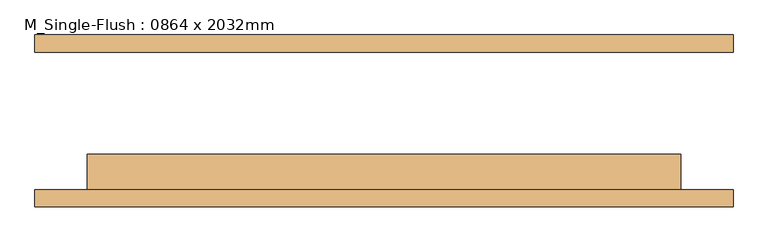
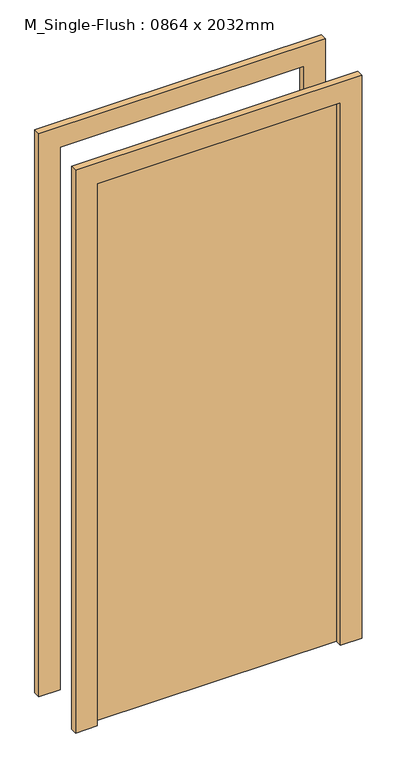
"""IFC4 building model written with IfcOpenShell, lengths in millimetres: door geometry, M_Single-Flush : 0864 x 2032mm."""

from ifc_helpers import new_model, si_unit, frame, origin, origin_with_axes, place, context, project, spatial, polyline, outline, extrude, source, transform, mapped, element, save


def m_single_flush_0864_x_2032mm_0516f16c(model_context):
    return source(origin(), model_context, "Body", "SweptSolid", [
        extrude(outline(polyline([(2108.0, -508.0), (0.0, -508.0), (0.0, -432.0), (2032.0, -432.0), (2032.0, 432.0), (0.0, 432.0), (0.0, 508.0), (2108.0, 508.0), (2108.0, -508.0)])), frame((0.0, -125.0, 0.0), z_axis=(0.0, 1.0, 0.0), x_axis=(0.0, 0.0, 1.0)), (0.0, 0.0, 1.0), 25.0),
        extrude(outline(polyline([(2108.0, 508.0), (2108.0, -508.0), (0.0, -508.0), (0.0, -432.0), (2032.0, -432.0), (2032.0, 432.0), (0.0, 432.0), (0.0, 508.0), (2108.0, 508.0)])), frame((0.0, 100.0, 0.0), z_axis=(0.0, 1.0, 0.0), x_axis=(0.0, 0.0, 1.0)), (0.0, 0.0, 1.0), 25.0),
        extrude(outline(polyline([(432.0, -49.0), (432.0, -100.0), (-432.0, -100.0), (-432.0, -49.0), (432.0, -49.0)])), origin_with_axes(), (0.0, 0.0, 1.0), 2032.0),
    ])


if __name__ == "__main__":
    model = new_model("IFC4")
    model_context = context("Model", 3, world=origin())
    ifc_project = project(units=[si_unit("LENGTHUNIT", "METRE", prefix="MILLI")], contexts=[model_context])
    site = spatial("IfcSite", under=ifc_project)
    building = spatial("IfcBuilding", under=site)
    placement = place(None, origin())
    m_single_flush_0864_x_2032mm_shape = m_single_flush_0864_x_2032mm_0516f16c(model_context)
    element("IfcDoor", 1, ObjectType="M_Single-Flush : 0864 x 2032mm", at=placement, inside=building, context=model_context, shape_type="MappedRepresentation", body=[
        mapped(m_single_flush_0864_x_2032mm_shape, transform((0.0, 0.0, 0.0), x_axis=(1.0, 0.0, 0.0), y_axis=(0.0, 1.0, 0.0), z_axis=(0.0, 0.0, 1.0))),
    ])
    save(model, "model.ifc")

# Revit data of these elements
# Type "M_Single-Flush : 0864 x 2032mm"
#   Type Mark = "21"
#   Thickness = 51 mm
#   Height = 2032 mm
#   Trim Projection Ext = 25 mm
#   Trim Projection Int = 25 mm
#   Trim Width = 76 mm
#   Width = 864 mm
#   Door Material = Door - Panel
#   Frame Material = Door - Frame
#   Function = (empty or 0)
#   Wall Closure = (empty or 0)
# Element 1 (IfcDoor, "M_Single-Flush : 0864 x 2032mm")
#   Materials on its faces: "Door - Frame", "Door - Panel"
# Materials
#   "Door - Panel": class "Wood", colour RGB 114 82 51, transparency 0
#   "Door - Frame": colour RGB 153 76 43, transparency 0
